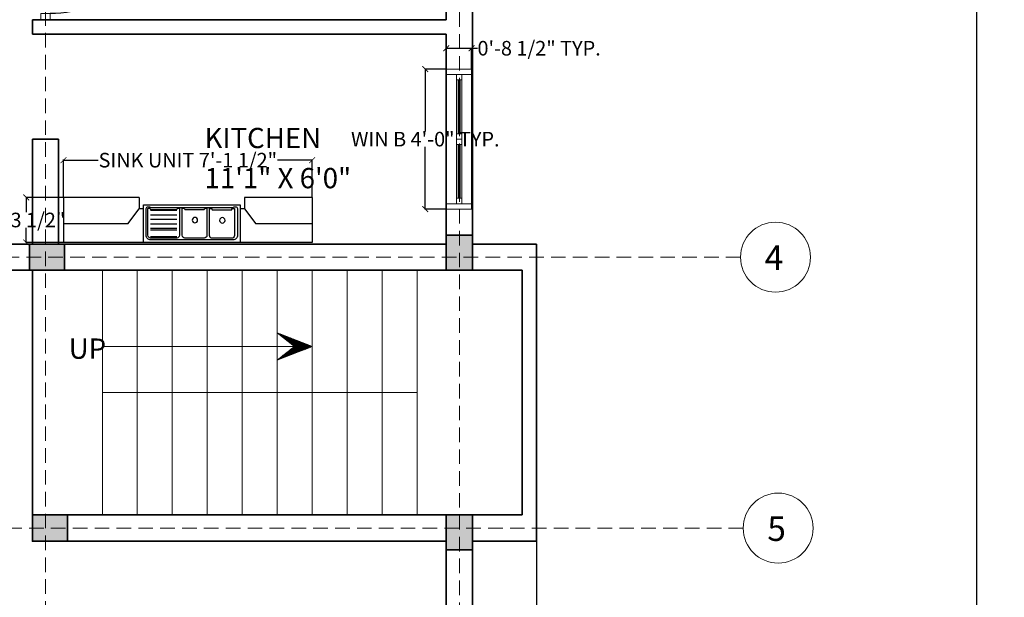
# Model space of a CAD drawing. Units: inches. Extents: x 782 to 2660, y -1008 to 166.
# Tile 5 of 12: x 1251 to 1589, y -598 to -400. Entities that reach past the tile are written whole.
import ezdxf

# ---------------------------------------------------------------- set-up
doc = ezdxf.new("R2010")
doc.units = ezdxf.units.IN
doc.header["$MEASUREMENT"] = 0
doc.linetypes.add('DASHED', pattern=[0.75, 0.5, -0.25])
for name, color, linetype, lineweight in [('A-ANNO-DIMS', 4, 'Continuous', 18), ('A-ANNO-SYMB', 4, 'Continuous', 18), ('A-ANNO-TEXT', 4, 'Continuous', 18), ('A-AREA-IDEN', 4, 'Continuous', 18), ('A-COLS', 7, 'Continuous', 35), ('A-Door', 150, 'Continuous', 18), ('A-FLOR-FIXT', 9, 'Continuous', 18), ('A-Glaz', 4, 'Continuous', 18), ('A-GRID', 8, 'DASHED', 13), ('A-GRID-IDEN', 7, 'Continuous', 18), ('A-WALL', 7, 'Continuous', 35), ('Stairs', 4, 'Continuous', 18)]:
    doc.layers.add(name, color=color, linetype=linetype, lineweight=lineweight)
doc.layers.add('NET 01', color=8, linetype='Continuous')
doc.layers.add('TEFRIS', color=11, linetype='Continuous')
doc.styles.get("Standard").update_dxf_attribs({"font": 'arial.ttf'})
doc.dimstyles.get("Standard").update_dxf_attribs({"dimtxt": 5, "dimasz": 2, "dimexe": 0.18, "dimexo": 0.0625, "dimgap": 0.09, "dimtad": 0, "dimtih": 1, "dimtoh": 1, "dimdec": 0, "dimzin": 0, "dimdsep": 46, "dimlunit": 3, "dimtxsty": 'Standard', "dimblk": 'ARCHTICK', "dimcen": 0.09, "dimadec": 0, "dimazin": 0, "dimtfac": 1, "dimtdec": 0, "dimtofl": 0, "dimtmove": 0, "dimatfit": 3, "dimfxl": 1, "dimtolj": 1, "dimtzin": 0, "dimarcsym": 0})

# ---------------------------------------------------------------- blocks, each defined once
blk = doc.blocks.new('A$C592222DF')
at = {"layer": 'A-Door'}
for points in [[(-0.0354, -0.0354), (-0.6718, 0.601), (-0.6364, 0.6364), (0, 0)], [(-0.95, 0), (-0.95, -0.075), (-0.9, -0.075), (-0.9, 0)], [(0, 0), (0, -0.075), (0.05, -0.075), (0.05, 0)]]:
    blk.add_lwpolyline(points, close=True, dxfattribs=at)
at = {"layer": 'NET 01'}
blk.add_arc((0, 0), 0.9, 135, 180, dxfattribs=at)
blk = doc.blocks.new('A$C5E722230')
at = {"layer": 'TEFRIS'}
for p, q in [((-0.6, -1.008), (-0.6, 0)), ((-0.6, 0), (0, 0)), ((-0.25, -0.858), (-0.25, 0)), ((0, -3.308), (0, 0)), ((-0.25, -0.858), (-0.45, -1.008)), ((-0.6, -1.008), (-0.45, -1.008)), ((-0.096, -1.124), (-0.454, -1.124)), ((-0.44, -1.16), (-0.44, -1.506)), ((-0.43, -1.16), (-0.43, -1.506)), ((-0.37, -1.16), (-0.37, -1.506)), ((-0.31, -1.16), (-0.31, -1.506)), ((-0.25, -1.16), (-0.25, -1.506)), ((-0.19, -1.16), (-0.19, -1.506)), ((-0.17, -1.16), (-0.17, -1.506)), ((-0.08, -1.16), (-0.08, -1.506)), ((-0.06, -1.506), (-0.06, -1.16)), ((-0.454, -1.542), (-0.096, -1.542)), ((-0.096, -1.579), (-0.454, -1.579)), ((-0.44, -1.615), (-0.44, -1.873)), ((-0.06, -1.873), (-0.06, -1.615)), ((-0.454, -1.909), (-0.096, -1.909)), ((-0.093, -1.943), (-0.451, -1.943)), ((-0.437, -1.979), (-0.437, -2.238)), ((-0.057, -2.238), (-0.057, -1.979)), ((-0.451, -2.274), (-0.093, -2.274)), ((-0.6, -3.308), (-0.6, -2.408)), ((-0.6, -2.408), (-0.45, -2.408)), ((-0.45, -2.408), (-0.25, -2.558)), ((-0.25, -3.308), (-0.25, -2.558)), ((-0.6, -3.308), (0, -3.308))]:
    blk.add_line(p, q, dxfattribs=at)
for points in [[(-0.45, -1.064), (-0.45, -1.008)], [(-0.45, -2.408), (-0.45, -2.353)]]:
    blk.add_lwpolyline(points, dxfattribs=at)
blk.add_lwpolyline([(0, -1.064), (-0.5, -1.064), (-0.5, -2.353), (0, -2.353)], close=True, dxfattribs=at)
blk.add_lwpolyline([(-0.096, -1.1), (-0.454, -1.1, 0.577816), (-0.464, -1.16), (-0.464, -2.257, 0.577816), (-0.454, -2.317), (-0.096, -2.317, 0.414214), (-0.036, -2.257), (-0.036, -1.16, 0.414214)], format="xyb", close=True, dxfattribs=at)
for centre in [(-0.298, -1.749), (-0.295, -2.114)]:
    blk.add_circle(centre, 0.036, dxfattribs=at)
for centre, radius, start, end in [((-0.435, -1.137), 0.023, 143.9853, 258.5157), ((-0.096, -1.16), 0.036, 0, 90), ((-0.435, -1.529), 0.023, 101.4843, 216.0147), ((-0.096, -1.506), 0.036, 270, 0), ((-0.435, -1.592), 0.023, 143.9853, 258.5157), ((-0.096, -1.615), 0.036, 0, 90), ((-0.435, -1.896), 0.023, 101.4843, 216.0147), ((-0.432, -1.957), 0.023, 143.9853, 258.5157), ((-0.096, -1.873), 0.036, 270, 0), ((-0.093, -1.979), 0.036, 0, 90), ((-0.432, -2.26), 0.023, 101.4843, 216.0147), ((-0.093, -2.238), 0.036, 270, 0)]:
    blk.add_arc(centre, radius, start, end, dxfattribs=at)
blk = doc.blocks.new('WIN-48-FRAME-B')
for p, q in [((8.69, 48), (0, 48)), ((0, 48), (0, 46.15)), ((8.69, 48), (0, 48)), ((8.69, 0), (8.69, 48)), ((8.69, 46.15), (8.69, 48)), ((0, 46.15), (8.69, 46.15)), ((0, 46.15), (8.69, 46.15)), ((0, 1.85), (0, 46.15)), ((3.5, 46.15), (3.5, 1.85)), ((3.5, 44.31), (5.35, 44.31)), ((4.05, 44.31), (4.05, 25.85)), ((4.42, 44.31), (4.42, 25.85)), ((4.79, 44.31), (4.79, 25.85)), ((5.35, 46.15), (5.35, 1.85)), ((5.35, 25.85), (3.5, 25.85)), ((5.35, 24), (3.5, 24)), ((5.35, 22.15), (3.5, 22.15)), ((4.05, 3.69), (4.05, 22.15)), ((4.42, 3.69), (4.42, 22.15)), ((4.79, 3.69), (4.79, 22.15)), ((3.5, 3.69), (5.35, 3.69)), ((0, 1.85), (8.69, 1.85)), ((0, 0), (0, 1.85)), ((0, 1.85), (8.69, 1.85)), ((0, 1.85), (8.69, 1.85)), ((8.69, 0), (0, 0)), ((0, 0), (8.69, 0)), ((8.69, 1.85), (8.69, 0))]:
    blk.add_line(p, q)
blk = doc.blocks.new('COL-9X12')
h = blk.add_hatch(color=256)
h.dxf.hatch_style = 1
h.paths.add_polyline_path([(9, 12), (0, 12), (0, 0), (9, 0)])
blk.add_lwpolyline([(0, 12), (9, 12), (9, 0), (0, 0)], close=True)
blk = doc.blocks.new('STAIR-TRAVEL-ARROW')
h = blk.add_hatch()
h.set_pattern_fill('ANSI31', color=256)
h.set_pattern_definition([(45, (-1279.684, 516.831), (-0.088388348, 0.088388348), [])])
h.paths.add_polyline_path([(60, 9.41), (65.9, 4.71), (60, 0), (72, 4.71)])
for p, q in [((65.9, 4.71), (60, 9.41)), ((60, 9.41), (72, 4.71)), ((0, 4.71), (65.9, 4.71)), ((65.9, 4.71), (60, 0)), ((60, 0), (72, 4.71))]:
    blk.add_line(p, q)
blk = doc.blocks.new('_ArchTick')
at = {"color": 0, "linetype": 'ByBlock', "const_width": 0.15}
blk.add_lwpolyline([(-0.5, -0.5), (0.5, 0.5)], dxfattribs=at)
blk = doc.blocks.new('*D37')
at = {"layer": 'A-ANNO-DIMS', "color": 0, "lineweight": -2, "transparency": 16777216}
for p, q in [((1397.62, -416.99), (1390.3, -416.99)), ((1390.48, -416.99), (1390.48, -438.35)), ((1390.48, -464.99), (1390.48, -443.64)), ((1397.62, -464.99), (1390.3, -464.99))]:
    blk.add_line(p, q, dxfattribs=at)
at = {"layer": 'Defpoints', "color": 0, "transparency": 16777216}
for p in [(1390.48, -416.99), (1397.68, -416.99), (1397.68, -464.99)]:
    blk.add_point(p, dxfattribs=at)
at = {"layer": 'A-ANNO-DIMS', "color": 0, "lineweight": -2, "transparency": 16777216, "xscale": 2, "yscale": 2, "zscale": 2}
for p, rotation in [((1390.48, -416.99), 90), ((1390.48, -464.99), 270)]:
    blk.add_blockref('_ArchTick', p, dxfattribs=dict(at, rotation=rotation))
at = {"layer": 'A-ANNO-DIMS', "color": 0, "transparency": 16777216, "insert": (1390.48, -440.99), "char_height": 5, "attachment_point": 5}
blk.add_mtext('\\A1;WIN B 4\'-0" TYP.', dxfattribs=at)
blk = doc.blocks.new('*D38')
at = {"layer": 'A-ANNO-DIMS', "color": 0, "lineweight": -2, "transparency": 16777216}
for p, q in [((1397.68, -416.93), (1397.68, -409.61)), ((1397.68, -409.79), (1406.38, -409.79)), ((1406.38, -416.93), (1406.38, -409.61)), ((1406.38, -409.79), (1408.38, -409.79))]:
    blk.add_line(p, q, dxfattribs=at)
at = {"layer": 'Defpoints', "color": 0, "transparency": 16777216}
for p in [(1406.38, -409.79), (1397.68, -416.99), (1406.38, -416.99)]:
    blk.add_point(p, dxfattribs=at)
at = {"layer": 'A-ANNO-DIMS', "color": 0, "lineweight": -2, "transparency": 16777216, "xscale": 2, "yscale": 2, "zscale": 2, "rotation": 180}
blk.add_blockref('_ArchTick', (1397.68, -409.79), dxfattribs=at)
at = {"layer": 'A-ANNO-DIMS', "color": 0, "lineweight": -2, "transparency": 16777216, "xscale": 2, "yscale": 2, "zscale": 2}
blk.add_blockref('_ArchTick', (1406.38, -409.79), dxfattribs=at)
at = {"layer": 'A-ANNO-DIMS', "color": 0, "transparency": 16777216, "insert": (1429.53, -409.79), "char_height": 5, "attachment_point": 5}
blk.add_mtext('\\A1;0\'-8 1/2" TYP.', dxfattribs=at)
blk = doc.blocks.new('*D47')
at = {"layer": 'A-ANNO-DIMS', "color": 0, "lineweight": -2, "transparency": 16777216}
for p, q in [((1266.35, -460.94), (1266.35, -448.03)), ((1266.35, -448.21), (1278.22, -448.21)), ((1351.66, -448.21), (1339.8, -448.21)), ((1351.66, -460.94), (1351.66, -448.03))]:
    blk.add_line(p, q, dxfattribs=at)
at = {"layer": 'Defpoints', "color": 0, "transparency": 16777216}
for p in [(1266.35, -448.21), (1266.35, -461), (1351.66, -461)]:
    blk.add_point(p, dxfattribs=at)
at = {"layer": 'A-ANNO-DIMS', "color": 0, "lineweight": -2, "transparency": 16777216, "xscale": 2, "yscale": 2, "zscale": 2, "rotation": 180}
blk.add_blockref('_ArchTick', (1266.35, -448.21), dxfattribs=at)
at = {"layer": 'A-ANNO-DIMS', "color": 0, "lineweight": -2, "transparency": 16777216, "xscale": 2, "yscale": 2, "zscale": 2}
blk.add_blockref('_ArchTick', (1351.66, -448.21), dxfattribs=at)
at = {"layer": 'A-ANNO-DIMS', "color": 0, "transparency": 16777216, "insert": (1309.01, -448.21), "char_height": 5, "attachment_point": 5}
blk.add_mtext('\\A1;SINK UNIT 7\'-1 1/2"', dxfattribs=at)
blk = doc.blocks.new('*D48')
at = {"layer": 'A-ANNO-DIMS', "color": 0, "lineweight": -2, "transparency": 16777216}
for p, q in [((1266.29, -461), (1253.38, -461)), ((1253.56, -461), (1253.56, -466.06)), ((1253.56, -476.47), (1253.56, -471.42)), ((1266.29, -476.47), (1253.38, -476.47))]:
    blk.add_line(p, q, dxfattribs=at)
at = {"layer": 'Defpoints', "color": 0, "transparency": 16777216}
for p in [(1266.35, -461), (1253.56, -476.47), (1266.35, -476.47)]:
    blk.add_point(p, dxfattribs=at)
at = {"layer": 'A-ANNO-DIMS', "color": 0, "lineweight": -2, "transparency": 16777216, "xscale": 2, "yscale": 2, "zscale": 2}
for p, rotation in [((1253.56, -461), 90), ((1253.56, -476.47), 270)]:
    blk.add_blockref('_ArchTick', p, dxfattribs=dict(at, rotation=rotation))
at = {"layer": 'A-ANNO-DIMS', "color": 0, "transparency": 16777216, "insert": (1253.56, -468.74), "char_height": 5, "attachment_point": 5}
blk.add_mtext('\\A1;1\'-3 1/2"', dxfattribs=at)
blk = doc.blocks.new('*D51')
at = {"layer": 'A-ANNO-DIMS', "color": 0, "lineweight": -2, "transparency": 16777216}
for p, q in [((1406.75, 45.01), (1579.89, 45.01)), ((1579.71, 45.01), (1579.71, -327.35)), ((1579.71, -704.99), (1579.71, -332.64)), ((1406.75, -704.99), (1579.89, -704.99))]:
    blk.add_line(p, q, dxfattribs=at)
at = {"layer": 'Defpoints', "color": 0, "transparency": 16777216}
for p in [(1406.68, 45.01), (1579.71, 45.01), (1406.68, -704.99)]:
    blk.add_point(p, dxfattribs=at)
at = {"layer": 'A-ANNO-DIMS', "color": 0, "lineweight": -2, "transparency": 16777216, "xscale": 2, "yscale": 2, "zscale": 2}
for p, rotation in [((1579.71, 45.01), 90), ((1579.71, -704.99), 270)]:
    blk.add_blockref('_ArchTick', p, dxfattribs=dict(at, rotation=rotation))
at = {"layer": 'A-ANNO-DIMS', "color": 0, "transparency": 16777216, "insert": (1579.71, -329.99), "char_height": 5, "attachment_point": 5}
blk.add_mtext('\\A1;62\'-6"', dxfattribs=at)
blk = doc.blocks.new('*D53')
at = {"layer": 'A-ANNO-DIMS', "color": 0, "lineweight": -2, "transparency": 16777216}
for p, q in [((1406.68, -579.06), (1406.68, -1005.36)), ((1428.68, -579.06), (1428.68, -1005.36)), ((1406.68, -1005.18), (1409.24, -1005.18)), ((1428.68, -1005.18), (1426.13, -1005.18))]:
    blk.add_line(p, q, dxfattribs=at)
at = {"layer": 'Defpoints', "color": 0, "transparency": 16777216}
for p in [(1406.68, -578.99), (1428.68, -578.99), (1428.68, -1005.18)]:
    blk.add_point(p, dxfattribs=at)
at = {"layer": 'A-ANNO-DIMS', "color": 0, "lineweight": -2, "transparency": 16777216, "xscale": 2, "yscale": 2, "zscale": 2, "rotation": 180}
blk.add_blockref('_ArchTick', (1406.68, -1005.18), dxfattribs=at)
at = {"layer": 'A-ANNO-DIMS', "color": 0, "lineweight": -2, "transparency": 16777216, "xscale": 2, "yscale": 2, "zscale": 2}
blk.add_blockref('_ArchTick', (1428.68, -1005.18), dxfattribs=at)
at = {"layer": 'A-ANNO-DIMS', "color": 0, "transparency": 16777216, "insert": (1417.68, -1005.18), "char_height": 5, "attachment_point": 5}
blk.add_mtext('\\A1;1\'-10"', dxfattribs=at)

msp = doc.modelspace()

# ---------------------------------------------------------------- linework, layer by layer
at = {"layer": 'A-ANNO-SYMB'}
msp.add_line((1279.68, -512.13), (1279.68, -512.13), dxfattribs=at)
at = {"layer": 'A-GRID', "ltscale": 10}
for p, q in [((1260.18, 82.94), (1260.18, -927.11)), ((1402.18, 82.53), (1402.18, -937.14)), ((1498.64, -481.49), (854.73, -481.49)), ((1499.56, -574.49), (847.83, -574.49))]:
    msp.add_line(p, q, dxfattribs=at)
at = {"layer": 'A-GRID-IDEN'}
for centre in [(1510.64, -481.49), (1511.56, -574.49)]:
    msp.add_circle(centre, 12, dxfattribs=at)
at = {"layer": 'A-WALL'}
for p, q in [((1406.68, 45.01), (1406.68, -476.99)), ((1397.68, -289.99), (1397.68, -399.99)), ((1264.68, -399.99), (1255.68, -399.99)), ((1255.68, -399.99), (1255.68, -404.99)), ((1264.68, -399.99), (1397.68, -399.99)), ((1264.68, -404.99), (1255.68, -404.99)), ((1264.68, -404.99), (1397.68, -404.99)), ((1397.68, -404.99), (1397.68, -476.99)), ((1264.68, -440.99), (1255.68, -440.99)), ((1255.68, -440.99), (1255.68, -476.99)), ((1264.68, -440.99), (1264.68, -476.99)), ((1107.68, -476.99), (1255.68, -476.99)), ((1264.68, -476.99), (1397.68, -476.99)), ((1406.68, -476.99), (1428.68, -476.99)), ((1428.68, -476.99), (1428.68, -578.99)), ((1098.68, -485.99), (1406.68, -485.99)), ((1255.68, -485.99), (1255.68, -578.99)), ((1264.68, -485.99), (1423.68, -485.99)), ((1423.68, -485.99), (1423.68, -569.99)), ((1255.68, -569.99), (1423.68, -569.99)), ((1255.68, -578.99), (1397.68, -578.99)), ((1397.68, -578.99), (1397.68, -704.99)), ((1406.68, -578.99), (1428.68, -578.99)), ((1406.68, -704.99), (1406.68, -578.99)), ((1406.68, -704.99), (1406.68, -578.99))]:
    msp.add_line(p, q, dxfattribs=at)
at = {"layer": 'Stairs'}
for p, q in [((1279.68, -485.99), (1279.68, -569.99)), ((1291.68, -485.99), (1291.68, -569.99)), ((1303.68, -485.99), (1303.68, -569.99)), ((1315.68, -485.99), (1315.68, -569.99)), ((1327.68, -485.99), (1327.68, -569.99)), ((1339.68, -485.99), (1339.68, -569.99)), ((1351.68, -485.99), (1351.68, -569.99)), ((1363.68, -485.99), (1363.68, -569.99)), ((1375.68, -485.99), (1375.68, -569.99)), ((1387.68, -485.99), (1387.68, -569.99)), ((1387.68, -527.99), (1279.68, -527.99))]:
    msp.add_line(p, q, dxfattribs=at)

# ---------------------------------------------------------------- block references
at = {"layer": 'A-ANNO-SYMB'}
msp.add_blockref('STAIR-TRAVEL-ARROW', (1279.68, -516.83), dxfattribs=at)
at = {"layer": 'A-COLS'}
for p, rotation in [((1406.68, -473.99), 180), ((1254.67, -476.99), 270.0000000000012), ((1255.68, -569.99), 270.000000000001), ((1406.68, -569.99), 180)]:
    msp.add_blockref('COL-9X12', p, dxfattribs=dict(at, rotation=rotation))
at = {"layer": 'A-Door', "xscale": -42, "yscale": 42, "zscale": 42, "rotation": 270}
msp.add_blockref('A$C592222DF', (1261.76, -360.09), dxfattribs=at)
at = {"layer": 'A-FLOR-FIXT', "xscale": -25.78565866541411, "yscale": 25.78565866541411, "zscale": 25.78565866541411, "rotation": 90}
msp.add_blockref('A$C5E722230', (1266.35, -476.47), dxfattribs=at)
at = {"layer": 'A-Glaz'}
msp.add_blockref('WIN-48-FRAME-B', (1397.68, -464.99), dxfattribs=at)

# ---------------------------------------------------------------- texts
at = {"layer": 'A-ANNO-TEXT'}
msp.add_text('UP', height=6.958, dxfattribs=at).set_placement((1268.14, -516.37))
at = {"layer": 'A-AREA-IDEN'}
for s, height, p in [('KITCHEN', 6.958, (1314.74, -444.08)), ('11\'1" X 6\'0"', 6.9576, (1314.74, -457.85))]:
    msp.add_text(s, height=height, dxfattribs=at).set_placement(p)
at = {"layer": 'A-GRID-IDEN'}
for s, p in [('4', (1506.91, -485.89)), ('5', (1507.82, -578.89))]:
    msp.add_text(s, height=8.41, dxfattribs=at).set_placement(p)

# ---------------------------------------------------------------- dimensions: what is measured, and where the dimension line sits
at = {"layer": 'A-ANNO-DIMS'}
for base, p1, p2, angle, picture, middle in [((1579.71, 45.01), (1406.68, -704.99), (1406.68, 45.01), 90, '*D51', (1579.71, -329.99)), ((1253.56, -476.47), (1266.35, -461), (1266.35, -476.47), 270, '*D48', (1253.56, -468.74))]:
    dim = msp.add_linear_dim(base=base, p1=p1, p2=p2, angle=angle, dimstyle='Standard', override={"dimdec": 1, "dimlfac": 1, "dimrnd": 0, "dimzin": 1, "dimdsep": 46, "dimlunit": 4, "dimfrac": 2}, dxfattribs=at)
    dim.commit()
    dim.dimension.update_dxf_attribs({"geometry": picture, "text_midpoint": middle})
dim = msp.add_linear_dim(base=(1406.38, -409.79), p1=(1397.68, -416.99), p2=(1406.38, -416.99), text='<> TYP.', dimstyle='Standard', override={"dimdec": 1, "dimlfac": 1, "dimrnd": 0, "dimzin": 1, "dimdsep": 46, "dimlunit": 4, "dimfrac": 2}, dxfattribs=at)
dim.commit()
dim.dimension.update_dxf_attribs({"geometry": '*D38', "text_midpoint": (1429.53, -409.79)})
for base, p1, p2, angle, text, picture, middle in [((1390.48, -416.99), (1397.68, -464.99), (1397.68, -416.99), 90, 'WIN B <> TYP.', '*D37', (1390.48, -440.99)), ((1266.35, -448.21), (1351.66, -461), (1266.35, -461), 180, 'SINK UNIT <>', '*D47', (1309.01, -448.21))]:
    dim = msp.add_linear_dim(base=base, p1=p1, p2=p2, angle=angle, text=text, dimstyle='Standard', override={"dimdec": 1, "dimlfac": 1, "dimrnd": 0, "dimzin": 1, "dimdsep": 46, "dimlunit": 4, "dimfrac": 2}, dxfattribs=at)
    dim.commit()
    dim.dimension.update_dxf_attribs({"geometry": picture, "text_midpoint": middle})
dim = msp.add_linear_dim(base=(1428.68, -1005.18), p1=(1406.68, -578.99), p2=(1428.68, -578.99), dimstyle='Standard', override={"dimdec": 1, "dimlfac": 1, "dimrnd": 0, "dimzin": 1, "dimdsep": 46, "dimlunit": 4, "dimfrac": 2}, dxfattribs=at)
dim.commit()
dim.dimension.update_dxf_attribs({"geometry": '*D53', "text_midpoint": (1417.68, -1005.18)})

doc.saveas('drawing.dxf')
